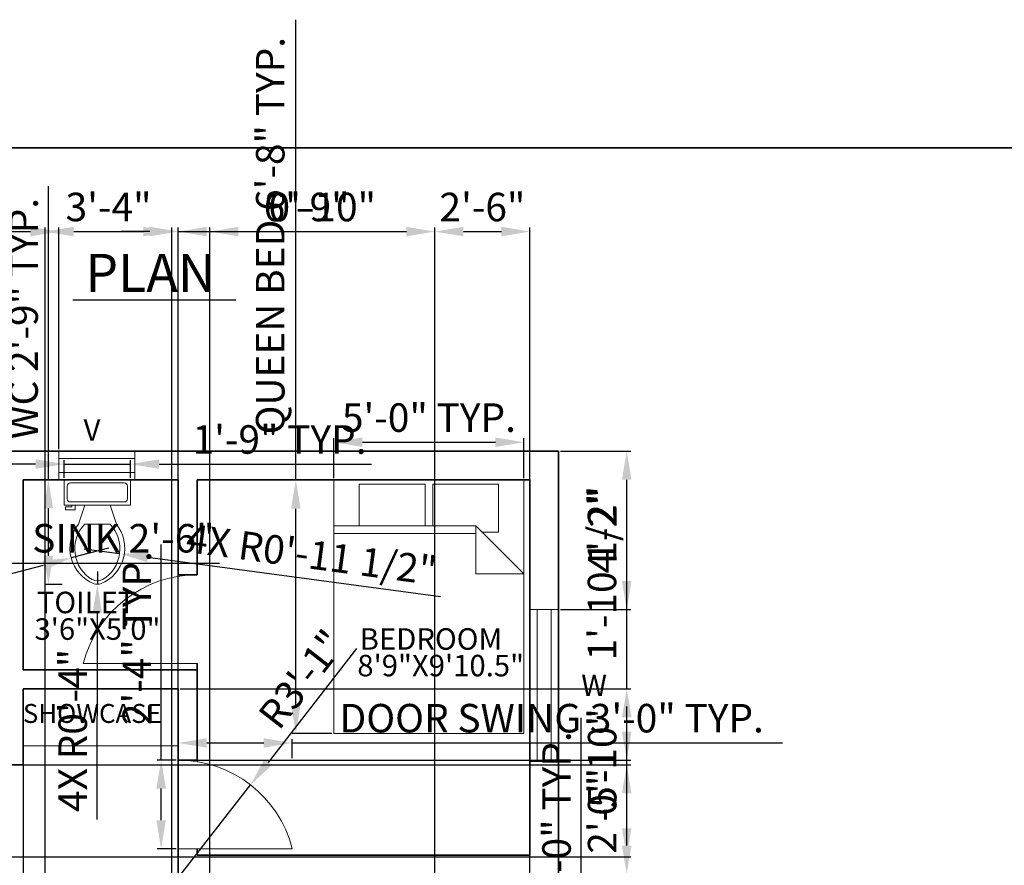
# Model space of a CAD drawing. Units: inches. Extents: x 1838 to 3181, y 1882 to 2430.
# Tile 3 of 4: x 2073 to 2384, y 2163 to 2430. Entities that reach past the tile are written whole.
import ezdxf

# ---------------------------------------------------------------- set-up
doc = ezdxf.new("R2010")
doc.units = ezdxf.units.IN
doc.linetypes.add('ACAD_ISO02W100', pattern=[15, 12, -3])
for name, color, linetype, lineweight in [('A-ANNO-TEXT', 7, 'Continuous', 18), ('A-ANNO-TITL', 6, 'Continuous', 25), ('A-ANNO-TTLB', 7, 'Continuous', 35), ('A-AREA-IDEN', 7, 'Continuous', 18), ('A-DOOR', 4, 'Continuous', 18), ('A-FLOR-CASE', 8, 'Continuous', 18), ('A-FLOR-FIXT', 9, 'Continuous', 18), ('A-FURN', 8, 'Continuous', 18), ('A-GLAZ', 11, 'Continuous', 18), ('A-WALL', 7, 'Continuous', 35), ('A-WALL-OVHD', 7, 'ACAD_ISO02W100', 18), ('S-ANNO-DIMS', 2, 'Continuous', 18)]:
    doc.layers.add(name, color=color, linetype=linetype, lineweight=lineweight)
doc.styles.get("Standard").update_dxf_attribs({"font": 'arial.ttf'})
doc.dimstyles.new('ISO-25', dxfattribs={"dimtxt": 9, "dimasz": 9, "dimexe": 1.25, "dimexo": 0.625, "dimgap": 2, "dimtad": 1, "dimdec": 1, "dimlunit": 4, "dimtxsty": 'Standard', "dimcen": 2.5, "dimadec": 0, "dimazin": 0, "dimtfac": 1, "dimtdec": 1, "dimtmove": 0, "dimatfit": 3, "dimfxl": 1, "dimarcsym": 0})

# ---------------------------------------------------------------- blocks, each defined once
blk = doc.blocks.new('Bed - Queen')
for p, q in [((0, -80.00003), (0, 0)), ((0, 0), (59.99999, 0)), ((59.99999, 0), (59.99999, -80.00003)), ((7.99999, -1.2), (28.79998, -1.2)), ((7.99999, -14.4), (7.99999, -1.2)), ((28.79998, -1.2), (28.79998, -14.4)), ((31.19999, -1.2), (51.99999, -1.2)), ((31.19999, -14.4), (31.19999, -1.2)), ((51.99999, -1.2), (51.99999, -16.4)), ((0, -14.4), (44.8, -14.4)), ((59.99999, -29.6), (44.8, -14.4)), ((44.8, -14.4), (44.8, -29.6)), ((44.8, -16.8), (0, -16.8)), ((51.99999, -16.4), (46.79936, -16.4)), ((44.8, -29.6), (59.99999, -29.6)), ((59.99999, -80.00003), (0, -80.00003))]:
    blk.add_line(p, q)
blk = doc.blocks.new('Toilet - top')
for p, q in [((9.5, -6), (9.5, -2)), ((-10, -8.5), (-8, -8.5)), ((-10, -9.5), (-10, -8.5)), ((-8, -8.5), (-8, -8)), ((-7, -8), (-7, -9.5)), ((-4, -8), (-6, -14)), ((4, -8), (6, -14)), ((-7, -9.5), (-10, -9.5)), ((4, -14), (-4, -14))]:
    blk.add_line(p, q)
blk.add_lwpolyline([(10.5, -8), (10.5, 0), (-10.5, 0), (-10.5, -8)], close=True)
for points in [[(-9.5, -2), (-9.5, -6)], [(8.5, -1), (-8.5, -1)], [(-8.5, -7), (8.5, -7)]]:
    blk.add_lwpolyline(points)
for centre, radius, start, end in [((-8.62, -1.88), 0.884, 81.8699, 188.1301), ((8.62, -1.88), 0.884, 351.8699, 98.1301), ((-8.62, -6.12), 0.884, 171.8699, 278.1301), ((8.62, -6.12), 0.884, 261.8699, 8.1301), ((3.52, -21.58), 12.17, 141.4691, 247.9714), ((4.2, -21.82), 11.33, 136.3677, 238.9468), ((-3.52, -21.58), 12.17, 292.0284, 38.5307), ((-4.2, -21.82), 11.33, 301.053, 43.6321), ((0, -27.88), 4, 245.7318, 294.2682), ((0, -29), 4, 254.8605, 285.1395)]:
    blk.add_arc(centre, radius, start, end)
blk = doc.blocks.new('WIN-48')
for p, q in [((0, 48), (9, 48)), ((2.25, 48), (2.25, 0)), ((6.75, 48), (6.75, 0)), ((0, 0), (9, 0))]:
    blk.add_line(p, q)
blk = doc.blocks.new('VENT-24')
for p, q in [((0, 24), (9, 24)), ((2.25, 24), (2.25, 0)), ((6.75, 24), (6.75, 0)), ((0, 0), (9, 0))]:
    blk.add_line(p, q)
blk = doc.blocks.new('DOOR-SWING-36')
blk.add_line((0, 0), (36, 0))
blk.add_arc((0, -9.14), 37.14, 14.25, 90)
blk = doc.blocks.new('*D23')
at = {"layer": 'Defpoints', "color": 0, "transparency": 16777216}
for p in [(2243.53, 2082.46), (2250.73, 2082.46), (2243.53, 2034.46)]:
    blk.add_point(p, dxfattribs=at)
at = {"layer": 'S-ANNO-DIMS', "color": 0, "lineweight": -2, "transparency": 16777216}
for p, q in [((2250.73, 2082.46), (2250.73, 2209.34)), ((2244.16, 2082.46), (2251.98, 2082.46)), ((2250.73, 2043.46), (2250.73, 2073.46)), ((2244.16, 2034.46), (2251.98, 2034.46))]:
    blk.add_line(p, q, dxfattribs=at)
at = {"layer": 'S-ANNO-DIMS', "color": 0, "transparency": 16777216}
for points in [[(2249.23, 2073.46), (2252.23, 2073.46), (2250.73, 2082.46)], [(2249.23, 2043.46), (2252.23, 2043.46), (2250.73, 2034.46)]]:
    blk.add_solid(points, dxfattribs=at)
at = {"layer": 'S-ANNO-DIMS', "color": 0, "transparency": 16777216, "insert": (2244.08, 2150.4), "char_height": 9, "attachment_point": 5, "rotation": 90}
blk.add_mtext('WINDOW 4\'-0" TYP.', dxfattribs=at)
blk = doc.blocks.new('*D27')
at = {"layer": 'Defpoints', "color": 0, "transparency": 16777216}
for p in [(2159.53, 2201.36), (2123.53, 2195.96), (2159.53, 2195.96)]:
    blk.add_point(p, dxfattribs=at)
at = {"layer": 'S-ANNO-DIMS', "color": 0, "lineweight": -2, "transparency": 16777216}
for p, q in [((2123.53, 2196.58), (2123.53, 2202.61)), ((2132.53, 2201.36), (2150.53, 2201.36)), ((2159.53, 2196.58), (2159.53, 2202.61)), ((2159.53, 2201.36), (2314.26, 2201.36))]:
    blk.add_line(p, q, dxfattribs=at)
at = {"layer": 'S-ANNO-DIMS', "color": 0, "transparency": 16777216}
for points in [[(2132.53, 2202.86), (2132.53, 2199.86), (2123.53, 2201.36)], [(2150.53, 2202.86), (2150.53, 2199.86), (2159.53, 2201.36)]]:
    blk.add_solid(points, dxfattribs=at)
at = {"layer": 'S-ANNO-DIMS', "color": 0, "transparency": 16777216, "insert": (2241.4, 2208.02), "char_height": 9, "attachment_point": 5}
blk.add_mtext('DOOR SWING 3\'-0" TYP.', dxfattribs=at)
blk = doc.blocks.new('*D28')
at = {"layer": 'Defpoints', "color": 0, "transparency": 16777216}
for p in [(2118.13, 2195.96), (2123.53, 2195.96), (2123.53, 2167.96)]:
    blk.add_point(p, dxfattribs=at)
at = {"layer": 'S-ANNO-DIMS', "color": 0, "lineweight": -2, "transparency": 16777216}
for p, q in [((2118.13, 2195.96), (2118.13, 2263.97)), ((2122.91, 2195.96), (2116.88, 2195.96)), ((2118.13, 2176.96), (2118.13, 2186.96)), ((2122.91, 2167.96), (2116.88, 2167.96))]:
    blk.add_line(p, q, dxfattribs=at)
at = {"layer": 'S-ANNO-DIMS', "color": 0, "transparency": 16777216}
for points in [[(2116.63, 2186.96), (2119.63, 2186.96), (2118.13, 2195.96)], [(2116.63, 2176.96), (2119.63, 2176.96), (2118.13, 2167.96)]]:
    blk.add_solid(points, dxfattribs=at)
at = {"layer": 'S-ANNO-DIMS', "color": 0, "transparency": 16777216, "insert": (2111.61, 2234.46), "char_height": 9, "attachment_point": 5, "rotation": 90}
blk.add_mtext('2\'-4" TYP.', dxfattribs=at)
blk = doc.blocks.new('*D29')
at = {"layer": 'Defpoints', "color": 0, "transparency": 16777216}
for p in [(2160.65, 2284.32), (2172.65, 2284.32), (2172.65, 2204.32)]:
    blk.add_point(p, dxfattribs=at)
at = {"layer": 'S-ANNO-DIMS', "color": 0, "lineweight": -2, "transparency": 16777216}
for p, q in [((2160.65, 2284.32), (2160.65, 2429.71)), ((2172.02, 2284.32), (2159.4, 2284.32)), ((2160.65, 2213.32), (2160.65, 2275.32)), ((2172.02, 2204.32), (2159.4, 2204.32))]:
    blk.add_line(p, q, dxfattribs=at)
at = {"layer": 'S-ANNO-DIMS', "color": 0, "transparency": 16777216}
for points in [[(2159.15, 2275.32), (2162.15, 2275.32), (2160.65, 2284.32)], [(2159.15, 2213.32), (2162.15, 2213.32), (2160.65, 2204.32)]]:
    blk.add_solid(points, dxfattribs=at)
at = {"layer": 'S-ANNO-DIMS', "color": 0, "transparency": 16777216, "insert": (2153.72, 2361.52), "char_height": 9, "attachment_point": 5, "rotation": 90}
blk.add_mtext('QUEEN BED 6\'-8" TYP.', dxfattribs=at)
blk = doc.blocks.new('*D30')
at = {"layer": 'Defpoints', "color": 0, "transparency": 16777216}
for p in [(2232.65, 2296.32), (2172.65, 2284.32), (2232.65, 2284.32)]:
    blk.add_point(p, dxfattribs=at)
at = {"layer": 'S-ANNO-DIMS', "color": 0, "lineweight": -2, "transparency": 16777216}
for p, q in [((2172.65, 2284.95), (2172.65, 2297.57)), ((2232.65, 2284.95), (2232.65, 2297.57)), ((2181.65, 2296.32), (2223.65, 2296.32))]:
    blk.add_line(p, q, dxfattribs=at)
at = {"layer": 'S-ANNO-DIMS', "color": 0, "transparency": 16777216}
for points in [[(2181.65, 2297.82), (2181.65, 2294.82), (2172.65, 2296.32)], [(2223.65, 2297.82), (2223.65, 2294.82), (2232.65, 2296.32)]]:
    blk.add_solid(points, dxfattribs=at)
at = {"layer": 'S-ANNO-DIMS', "color": 0, "transparency": 16777216, "insert": (2202.65, 2302.92), "char_height": 9, "attachment_point": 5}
blk.add_mtext('5\'-0" TYP.', dxfattribs=at)
blk = doc.blocks.new('*D31')
at = {"layer": 'Defpoints', "color": 0, "transparency": 16777216}
for p in [(2082.53, 2284.46), (2087.49, 2284.46), (2087.49, 2251.41)]:
    blk.add_point(p, dxfattribs=at)
at = {"layer": 'S-ANNO-DIMS', "color": 0, "lineweight": -2, "transparency": 16777216}
for p, q in [((2082.53, 2284.46), (2082.53, 2377.12)), ((2086.87, 2284.46), (2081.28, 2284.46)), ((2082.53, 2260.41), (2082.53, 2275.46)), ((2086.87, 2251.41), (2081.28, 2251.41))]:
    blk.add_line(p, q, dxfattribs=at)
at = {"layer": 'S-ANNO-DIMS', "color": 0, "transparency": 16777216}
for points in [[(2081.03, 2275.46), (2084.03, 2275.46), (2082.53, 2284.46)], [(2081.03, 2260.41), (2084.03, 2260.41), (2082.53, 2251.41)]]:
    blk.add_solid(points, dxfattribs=at)
at = {"layer": 'S-ANNO-DIMS', "color": 0, "transparency": 16777216, "insert": (2075.88, 2335.29), "char_height": 9, "attachment_point": 5, "rotation": 90}
blk.add_mtext('WC 2\'-9" TYP.', dxfattribs=at)
blk = doc.blocks.new('*D32')
at = {"layer": 'Defpoints', "color": 0, "transparency": 16777216}
for p in [(2108.49, 2289.41), (2087.49, 2284.46), (2108.49, 2284.46)]:
    blk.add_point(p, dxfattribs=at)
at = {"layer": 'S-ANNO-DIMS', "color": 0, "lineweight": -2, "transparency": 16777216}
for p, q in [((2087.49, 2285.08), (2087.49, 2290.66)), ((2108.49, 2285.08), (2108.49, 2290.66)), ((2078.49, 2289.41), (2069.49, 2289.41)), ((2087.49, 2289.41), (2108.49, 2289.41)), ((2117.49, 2289.41), (2184.5, 2289.41))]:
    blk.add_line(p, q, dxfattribs=at)
at = {"layer": 'S-ANNO-DIMS', "color": 0, "transparency": 16777216}
for points in [[(2078.49, 2290.91), (2078.49, 2287.91), (2087.49, 2289.41)], [(2117.49, 2290.91), (2117.49, 2287.91), (2108.49, 2289.41)]]:
    blk.add_solid(points, dxfattribs=at)
at = {"layer": 'S-ANNO-DIMS', "color": 0, "transparency": 16777216, "insert": (2155.5, 2296.01), "char_height": 9, "attachment_point": 5}
blk.add_mtext('1\'-9" TYP.', dxfattribs=at)
blk = doc.blocks.new('*D37')
at = {"layer": 'Defpoints', "color": 0, "transparency": 16777216}
for p in [(2036.86, 2262.67), (2066.86, 2262.67), (2066.86, 2258.17)]:
    blk.add_point(p, dxfattribs=at)
at = {"layer": 'S-ANNO-DIMS', "color": 0, "lineweight": -2, "transparency": 16777216}
for p, q in [((2036.86, 2262.04), (2036.86, 2256.92)), ((2066.86, 2262.04), (2066.86, 2256.92)), ((2045.86, 2258.17), (2057.86, 2258.17)), ((2066.86, 2258.17), (2136.58, 2258.17))]:
    blk.add_line(p, q, dxfattribs=at)
at = {"layer": 'S-ANNO-DIMS', "color": 0, "transparency": 16777216}
for points in [[(2045.86, 2259.67), (2045.86, 2256.67), (2036.86, 2258.17)], [(2057.86, 2259.67), (2057.86, 2256.67), (2066.86, 2258.17)]]:
    blk.add_solid(points, dxfattribs=at)
at = {"layer": 'S-ANNO-DIMS', "color": 0, "transparency": 16777216, "insert": (2106.22, 2264.82), "char_height": 9, "attachment_point": 5}
blk.add_mtext('SINK 2\'-6"', dxfattribs=at)
blk = doc.blocks.new('*D42')
at = {"layer": 'Defpoints', "color": 0, "transparency": 16777216}
for p in [(2002.53, 2194.46), (2265.08, 2194.46), (2002.53, 2165.46)]:
    blk.add_point(p, dxfattribs=at)
at = {"layer": 'S-ANNO-DIMS', "color": 0, "lineweight": -2, "transparency": 16777216}
for p, q in [((2003.16, 2194.46), (2266.33, 2194.46)), ((2265.08, 2174.46), (2265.08, 2185.46)), ((2003.16, 2165.46), (2266.33, 2165.46))]:
    blk.add_line(p, q, dxfattribs=at)
at = {"layer": 'S-ANNO-DIMS', "color": 0, "transparency": 16777216}
for points in [[(2263.58, 2185.46), (2266.58, 2185.46), (2265.08, 2194.46)], [(2263.58, 2174.46), (2266.58, 2174.46), (2265.08, 2165.46)]]:
    blk.add_solid(points, dxfattribs=at)
at = {"layer": 'S-ANNO-DIMS', "color": 0, "transparency": 16777216, "insert": (2258.49, 2179.96), "char_height": 9, "attachment_point": 5, "rotation": 90}
blk.add_mtext('2\'-5"', dxfattribs=at)
blk = doc.blocks.new('*D46')
at = {"layer": 'Defpoints', "color": 0, "transparency": 16777216}
for p in [(2234.53, 2159.96), (2265.08, 2159.96), (2234.53, 2149.73)]:
    blk.add_point(p, dxfattribs=at)
at = {"layer": 'S-ANNO-DIMS', "color": 0, "lineweight": -2, "transparency": 16777216}
for p, q in [((2265.08, 2168.96), (2265.08, 2212.87)), ((2235.16, 2159.96), (2266.33, 2159.96)), ((2265.08, 2149.73), (2265.08, 2159.96)), ((2235.16, 2149.73), (2266.33, 2149.73)), ((2265.08, 2140.73), (2265.08, 2131.73))]:
    blk.add_line(p, q, dxfattribs=at)
at = {"layer": 'S-ANNO-DIMS', "color": 0, "transparency": 16777216}
for points in [[(2263.58, 2168.96), (2266.58, 2168.96), (2265.08, 2159.96)], [(2263.58, 2140.73), (2266.58, 2140.73), (2265.08, 2149.73)]]:
    blk.add_solid(points, dxfattribs=at)
at = {"layer": 'S-ANNO-DIMS', "color": 0, "transparency": 16777216, "insert": (2258.49, 2195.41), "char_height": 9, "attachment_point": 5, "rotation": 90}
blk.add_mtext('0\'-10"', dxfattribs=at)
blk = doc.blocks.new('*D47')
at = {"layer": 'Defpoints', "color": 0, "transparency": 16777216}
for p in [(2243.53, 2293.46), (2265.08, 2293.46), (2243.53, 2243.46)]:
    blk.add_point(p, dxfattribs=at)
at = {"layer": 'S-ANNO-DIMS', "color": 0, "lineweight": -2, "transparency": 16777216}
for p, q in [((2244.16, 2293.46), (2266.33, 2293.46)), ((2265.08, 2252.46), (2265.08, 2284.46)), ((2244.16, 2243.46), (2266.33, 2243.46))]:
    blk.add_line(p, q, dxfattribs=at)
at = {"layer": 'S-ANNO-DIMS', "color": 0, "transparency": 16777216}
for points in [[(2263.58, 2284.46), (2266.58, 2284.46), (2265.08, 2293.46)], [(2263.58, 2252.46), (2266.58, 2252.46), (2265.08, 2243.46)]]:
    blk.add_solid(points, dxfattribs=at)
at = {"layer": 'S-ANNO-DIMS', "color": 0, "transparency": 16777216, "insert": (2258.57, 2268.46), "char_height": 9, "attachment_point": 5, "rotation": 90}
blk.add_mtext('4\'-2"', dxfattribs=at)
blk = doc.blocks.new('*D48')
at = {"layer": 'Defpoints', "color": 0, "transparency": 16777216}
for p in [(2085.84, 2362.82), (1993.53, 2293.46), (2085.84, 2293.46)]:
    blk.add_point(p, dxfattribs=at)
at = {"layer": 'S-ANNO-DIMS', "color": 0, "lineweight": -2, "transparency": 16777216}
for p, q in [((1993.53, 2294.08), (1993.53, 2364.07)), ((2002.53, 2362.82), (2076.84, 2362.82)), ((2085.84, 2294.08), (2085.84, 2364.07))]:
    blk.add_line(p, q, dxfattribs=at)
at = {"layer": 'S-ANNO-DIMS', "color": 0, "transparency": 16777216}
for points in [[(2002.53, 2364.32), (2002.53, 2361.32), (1993.53, 2362.82)], [(2076.84, 2364.32), (2076.84, 2361.32), (2085.84, 2362.82)]]:
    blk.add_solid(points, dxfattribs=at)
at = {"layer": 'S-ANNO-DIMS', "color": 0, "transparency": 16777216, "insert": (2039.69, 2369.47), "char_height": 9, "attachment_point": 5}
blk.add_mtext('7\'-8 1/2"', dxfattribs=at)
blk = doc.blocks.new('*D49')
at = {"layer": 'Defpoints', "color": 0, "transparency": 16777216}
for p in [(2133.53, 2362.82), (2123.53, 1939.46), (2133.53, 1939.46)]:
    blk.add_point(p, dxfattribs=at)
at = {"layer": 'S-ANNO-DIMS', "color": 0, "lineweight": -2, "transparency": 16777216}
for p, q in [((2114.53, 2362.82), (2105.53, 2362.82)), ((2123.53, 1940.08), (2123.53, 2364.07)), ((2123.53, 2362.82), (2133.53, 2362.82)), ((2133.53, 1940.08), (2133.53, 2364.07)), ((2142.53, 2362.82), (2186.45, 2362.82))]:
    blk.add_line(p, q, dxfattribs=at)
at = {"layer": 'S-ANNO-DIMS', "color": 0, "transparency": 16777216}
for points in [[(2114.53, 2364.32), (2114.53, 2361.32), (2123.53, 2362.82)], [(2142.53, 2364.32), (2142.53, 2361.32), (2133.53, 2362.82)]]:
    blk.add_solid(points, dxfattribs=at)
at = {"layer": 'S-ANNO-DIMS', "color": 0, "transparency": 16777216, "insert": (2168.99, 2369.41), "char_height": 9, "attachment_point": 5}
blk.add_mtext('0\'-10"', dxfattribs=at)
blk = doc.blocks.new('*D50')
at = {"layer": 'Defpoints', "color": 0, "transparency": 16777216}
for p in [(2204.53, 2362.82), (2123.53, 1999.46), (2204.53, 1999.46)]:
    blk.add_point(p, dxfattribs=at)
at = {"layer": 'S-ANNO-DIMS', "color": 0, "lineweight": -2, "transparency": 16777216}
for p, q in [((2123.53, 2000.08), (2123.53, 2364.07)), ((2132.53, 2362.82), (2195.53, 2362.82)), ((2204.53, 2000.08), (2204.53, 2364.07))]:
    blk.add_line(p, q, dxfattribs=at)
at = {"layer": 'S-ANNO-DIMS', "color": 0, "transparency": 16777216}
for points in [[(2132.53, 2364.32), (2132.53, 2361.32), (2123.53, 2362.82)], [(2195.53, 2364.32), (2195.53, 2361.32), (2204.53, 2362.82)]]:
    blk.add_solid(points, dxfattribs=at)
at = {"layer": 'S-ANNO-DIMS', "color": 0, "transparency": 16777216, "insert": (2164.03, 2369.41), "char_height": 9, "attachment_point": 5}
blk.add_mtext('6\'-9"', dxfattribs=at)
blk = doc.blocks.new('*D51')
at = {"layer": 'Defpoints', "color": 0, "transparency": 16777216}
for p in [(2234.53, 2362.82), (2204.53, 1999.46), (2234.53, 1999.46)]:
    blk.add_point(p, dxfattribs=at)
at = {"layer": 'S-ANNO-DIMS', "color": 0, "lineweight": -2, "transparency": 16777216}
for p, q in [((2204.53, 2000.08), (2204.53, 2364.07)), ((2213.53, 2362.82), (2225.53, 2362.82)), ((2234.53, 2000.08), (2234.53, 2364.07))]:
    blk.add_line(p, q, dxfattribs=at)
at = {"layer": 'S-ANNO-DIMS', "color": 0, "transparency": 16777216}
for points in [[(2213.53, 2364.32), (2213.53, 2361.32), (2204.53, 2362.82)], [(2225.53, 2364.32), (2225.53, 2361.32), (2234.53, 2362.82)]]:
    blk.add_solid(points, dxfattribs=at)
at = {"layer": 'S-ANNO-DIMS', "color": 0, "transparency": 16777216, "insert": (2219.53, 2369.41), "char_height": 9, "attachment_point": 5}
blk.add_mtext('2\'-6"', dxfattribs=at)
blk = doc.blocks.new('*D53')
at = {"layer": 'Defpoints', "color": 0, "transparency": 16777216}
for p in [(2121.53, 2362.82), (2081.53, 1999.46), (2121.53, 1999.46)]:
    blk.add_point(p, dxfattribs=at)
at = {"layer": 'S-ANNO-DIMS', "color": 0, "lineweight": -2, "transparency": 16777216}
for p, q in [((2081.53, 2000.08), (2081.53, 2364.07)), ((2090.53, 2362.82), (2112.53, 2362.82)), ((2121.53, 2000.08), (2121.53, 2364.07))]:
    blk.add_line(p, q, dxfattribs=at)
at = {"layer": 'S-ANNO-DIMS', "color": 0, "transparency": 16777216}
for points in [[(2090.53, 2364.32), (2090.53, 2361.32), (2081.53, 2362.82)], [(2112.53, 2364.32), (2112.53, 2361.32), (2121.53, 2362.82)]]:
    blk.add_solid(points, dxfattribs=at)
at = {"layer": 'S-ANNO-DIMS', "color": 0, "transparency": 16777216, "insert": (2101.53, 2369.42), "char_height": 9, "attachment_point": 5}
blk.add_mtext('3\'-4"', dxfattribs=at)
blk = doc.blocks.new('*D55')
at = {"layer": 'Defpoints', "color": 0, "transparency": 16777216}
for p in [(2068.53, 2194.46), (2074.53, 2194.46), (2074.53, 1908.91)]:
    blk.add_point(p, dxfattribs=at)
at = {"layer": 'S-ANNO-DIMS', "color": 0, "lineweight": -2, "transparency": 16777216}
for p, q in [((2068.53, 2193.83), (2068.53, 1907.66)), ((2074.53, 2193.83), (2074.53, 1907.66)), ((2059.53, 1908.91), (2050.53, 1908.91)), ((2068.53, 1908.91), (2074.53, 1908.91)), ((2083.53, 1908.91), (2120.46, 1908.91))]:
    blk.add_line(p, q, dxfattribs=at)
at = {"layer": 'S-ANNO-DIMS', "color": 0, "transparency": 16777216}
for points in [[(2059.53, 1910.41), (2059.53, 1907.41), (2068.53, 1908.91)], [(2083.53, 1910.41), (2083.53, 1907.41), (2074.53, 1908.91)]]:
    blk.add_solid(points, dxfattribs=at)
at = {"layer": 'S-ANNO-DIMS', "color": 0, "transparency": 16777216, "insert": (2106.5, 1915.5), "char_height": 9, "attachment_point": 5}
blk.add_mtext('0\'-6"', dxfattribs=at)
blk = doc.blocks.new('*D56')
at = {"layer": 'Defpoints', "color": 0, "transparency": 16777216}
for p in [(2074.53, 2218.46), (2123.53, 2218.46), (2123.53, 1908.91)]:
    blk.add_point(p, dxfattribs=at)
at = {"layer": 'S-ANNO-DIMS', "color": 0, "lineweight": -2, "transparency": 16777216}
for p, q in [((2074.53, 2217.83), (2074.53, 1907.66)), ((2123.53, 2217.83), (2123.53, 1907.66)), ((2083.53, 1908.91), (2114.53, 1908.91))]:
    blk.add_line(p, q, dxfattribs=at)
at = {"layer": 'S-ANNO-DIMS', "color": 0, "transparency": 16777216}
for points in [[(2083.53, 1910.41), (2083.53, 1907.41), (2074.53, 1908.91)], [(2114.53, 1910.41), (2114.53, 1907.41), (2123.53, 1908.91)]]:
    blk.add_solid(points, dxfattribs=at)
at = {"layer": 'S-ANNO-DIMS', "color": 0, "transparency": 16777216, "insert": (2099.03, 1915.42), "char_height": 9, "attachment_point": 5}
blk.add_mtext('4\'-1"', dxfattribs=at)
blk = doc.blocks.new('*D57')
at = {"layer": 'Defpoints', "color": 0, "transparency": 16777216}
for p in [(2123.53, 2218.46), (2265.08, 2218.46), (2123.53, 2195.96)]:
    blk.add_point(p, dxfattribs=at)
at = {"layer": 'S-ANNO-DIMS', "color": 0, "lineweight": -2, "transparency": 16777216}
for p, q in [((2265.08, 2218.46), (2265.08, 2282.5)), ((2124.16, 2218.46), (2266.33, 2218.46)), ((2265.08, 2204.96), (2265.08, 2209.46)), ((2124.16, 2195.96), (2266.33, 2195.96))]:
    blk.add_line(p, q, dxfattribs=at)
at = {"layer": 'S-ANNO-DIMS', "color": 0, "transparency": 16777216}
for points in [[(2263.58, 2209.46), (2266.58, 2209.46), (2265.08, 2218.46)], [(2263.58, 2204.96), (2266.58, 2204.96), (2265.08, 2195.96)]]:
    blk.add_solid(points, dxfattribs=at)
at = {"layer": 'S-ANNO-DIMS', "color": 0, "transparency": 16777216, "insert": (2258.43, 2254.98), "char_height": 9, "attachment_point": 5, "rotation": 90}
blk.add_mtext('1\'-10 1/2"', dxfattribs=at)
blk = doc.blocks.new('*D72')
at = {"layer": 'Defpoints', "color": 0, "transparency": 16777216}
for p in [(2146.34, 2188.13), (2123.53, 2158.81)]:
    blk.add_point(p, dxfattribs=at)
at = {"layer": 'S-ANNO-DIMS', "color": 0, "lineweight": -2, "transparency": 16777216}
for p, q in [((2179.82, 2231.18), (2151.86, 2195.24)), ((2123.53, 2158.81), (2146.34, 2188.13))]:
    blk.add_line(p, q, dxfattribs=at)
at = {"layer": 'S-ANNO-DIMS', "color": 0, "transparency": 16777216}
blk.add_solid([(2150.68, 2196.16), (2153.05, 2194.32), (2146.34, 2188.13)], dxfattribs=at)
at = {"layer": 'S-ANNO-DIMS', "color": 0, "transparency": 16777216, "insert": (2163.4, 2220.81), "char_height": 9, "attachment_point": 5, "rotation": 52.1256}
blk.add_mtext('R3\'-1"', dxfattribs=at)
blk = doc.blocks.new('*D74')
at = {"layer": 'Defpoints', "color": 0, "transparency": 16777216}
for p in [(2101.51, 2262.88), (2089.74, 2259.78)]:
    blk.add_point(p, dxfattribs=at)
at = {"layer": 'S-ANNO-DIMS', "color": 0, "lineweight": -2, "transparency": 16777216}
for p, q in [((2101.51, 2262.88), (2089.74, 2259.78)), ((2017.94, 2240.92), (2081.04, 2257.5))]:
    blk.add_line(p, q, dxfattribs=at)
at = {"layer": 'S-ANNO-DIMS', "color": 0, "transparency": 16777216}
blk.add_solid([(2080.65, 2258.95), (2081.42, 2256.05), (2089.74, 2259.78)], dxfattribs=at)
at = {"layer": 'S-ANNO-DIMS', "color": 0, "transparency": 16777216, "insert": (2043.46, 2254.44), "char_height": 9, "attachment_point": 5, "rotation": 14.7211}
blk.add_mtext('4X R1\'-0"', dxfattribs=at)
blk = doc.blocks.new('*D75')
at = {"layer": 'Defpoints', "color": 0, "transparency": 16777216}
for p in [(2093.79, 2262.64), (2105.02, 2261.13)]:
    blk.add_point(p, dxfattribs=at)
at = {"layer": 'S-ANNO-DIMS', "color": 0, "lineweight": -2, "transparency": 16777216}
for p, q in [((2093.79, 2262.64), (2105.02, 2261.13)), ((2206.31, 2247.51), (2113.94, 2259.93))]:
    blk.add_line(p, q, dxfattribs=at)
at = {"layer": 'S-ANNO-DIMS', "color": 0, "transparency": 16777216}
blk.add_solid([(2114.14, 2261.42), (2113.74, 2258.44), (2105.02, 2261.13)], dxfattribs=at)
at = {"layer": 'S-ANNO-DIMS', "color": 0, "transparency": 16777216, "insert": (2165.47, 2259.72), "char_height": 9, "attachment_point": 5, "rotation": 352.3432}
blk.add_mtext('4X R0\'-11 1/2"', dxfattribs=at)
blk = doc.blocks.new('*D76')
at = {"layer": 'Defpoints', "color": 0, "transparency": 16777216}
for p in [(2097.99, 2255.46), (2097.99, 2251.46)]:
    blk.add_point(p, dxfattribs=at)
at = {"layer": 'S-ANNO-DIMS', "color": 0, "lineweight": -2, "transparency": 16777216}
for p, q in [((2097.99, 2255.46), (2097.99, 2251.46)), ((2097.98, 2177.22), (2097.99, 2242.46))]:
    blk.add_line(p, q, dxfattribs=at)
at = {"layer": 'S-ANNO-DIMS', "color": 0, "transparency": 16777216}
blk.add_solid([(2096.49, 2242.46), (2099.49, 2242.46), (2097.99, 2251.46)], dxfattribs=at)
at = {"layer": 'S-ANNO-DIMS', "color": 0, "transparency": 16777216, "insert": (2091.39, 2205.34), "char_height": 9, "attachment_point": 5, "rotation": 89.9946}
blk.add_mtext('4X R0\'-4"', dxfattribs=at)

msp = doc.modelspace()

# ---------------------------------------------------------------- linework, layer by layer
at = {"layer": 'A-ANNO-TITL'}
msp.add_line((2090.21, 2341.27), (2141.65, 2341.27), dxfattribs=at)
at = {"layer": 'A-ANNO-TTLB'}
msp.add_lwpolyline([(1905.37, 2389.23), (3180.85, 2389.23), (3180.85, 1893.51), (1905.37, 1893.51)], close=True, dxfattribs=at)
at = {"layer": 'A-FLOR-CASE'}
msp.add_line((2074.53, 2200.46), (2123.53, 2200.46), dxfattribs=at)
at = {"layer": 'A-WALL'}
for p, q in [((1993.53, 2293.46), (2243.53, 2293.46)), ((2243.53, 2293.46), (2243.53, 1930.46)), ((2074.53, 2284.46), (2074.53, 2224.46)), ((2074.53, 2284.46), (2123.53, 2284.46)), ((2123.53, 2284.46), (2123.53, 2254.46)), ((2129.53, 2284.46), (2129.53, 2254.46)), ((2129.53, 2284.46), (2234.53, 2284.46)), ((2234.53, 2284.46), (2234.53, 2165.96)), ((2123.53, 2254.46), (2129.53, 2254.46)), ((2129.53, 2226.46), (2129.53, 2195.96)), ((2074.53, 2224.46), (2129.53, 2224.46)), ((2074.53, 2218.46), (2123.53, 2218.46)), ((2074.53, 2218.46), (2074.53, 2194.46)), ((2123.53, 2218.46), (2123.53, 2195.96)), ((2068.53, 2194.46), (2074.53, 2194.46)), ((2123.53, 2195.96), (2129.53, 2195.96)), ((2129.53, 2195.46), (2129.61, 2195.46)), ((2123.53, 2167.96), (2123.53, 2157.96)), ((2129.53, 2167.96), (2129.53, 2165.96)), ((2129.53, 2165.96), (2234.53, 2165.96))]:
    msp.add_line(p, q, dxfattribs=at)
at = {"layer": 'A-WALL-OVHD'}
msp.add_line((2030.53, 2194.46), (2074.53, 2194.46), dxfattribs=at)

# ---------------------------------------------------------------- block references
at = {"layer": 'A-DOOR', "extrusion": (0, 0, -1), "zscale": -1}
msp.add_blockref('DOOR-SWING-36', (-2129.53, 2226.46), dxfattribs=at)
at = {"layer": 'A-DOOR'}
msp.add_blockref('DOOR-SWING-36', (2123.53, 2167.96), dxfattribs=at)
at = {"layer": 'A-FLOR-FIXT'}
msp.add_blockref('Toilet - top', (2097.99, 2284.46), dxfattribs=at)
at = {"layer": 'A-FURN'}
msp.add_blockref('Bed - Queen', (2172.65, 2284.32), dxfattribs=at)
at = {"layer": 'A-GLAZ'}
for name, p, rotation in [('VENT-24', (2109.84, 2284.46), 90.00000000000641), ('WIN-48', (2243.53, 2243.46), 180)]:
    msp.add_blockref(name, p, dxfattribs=dict(at, rotation=rotation))

# ---------------------------------------------------------------- texts
at = {"layer": 'A-ANNO-TEXT'}
for s, height, p in [('V', 6.78, (2093.64, 2296.78)), ('W', 6.78, (2250.72, 2216.17)), ('SHOWCASE', 5.979, (2074.5, 2207.69))]:
    msp.add_text(s, height=height, dxfattribs=at).set_placement(p)
at = {"layer": 'A-ANNO-TITL'}
msp.add_text('PLAN', height=12, dxfattribs=at).set_placement((2094.19, 2343.79))
at = {"layer": 'A-AREA-IDEN'}
for s, height, p in [('TOILET', 6.784, (2078.88, 2242.33)), (' 3\'6"X5\'0"', 6.784, (2076.07, 2233.93)), ('BEDROOM', 6.784, (2180.78, 2230.8)), (' 8\'9"X9\'10.5"', 6.7841, (2177.97, 2222.4))]:
    msp.add_text(s, height=height, dxfattribs=at).set_placement(p)

# ---------------------------------------------------------------- dimensions: what is measured, and where the dimension line sits
at = {"layer": 'S-ANNO-DIMS'}
for base, p1, p2, text, picture, middle in [((2160.65, 2284.32), (2172.65, 2204.32), (2172.65, 2284.32), 'QUEEN BED <> TYP.', '*D29', (2153.72, 2361.52)), ((2082.5334, 2284.4559), (2087.4904, 2251.4097), (2087.4904, 2284.4559), 'WC <> TYP.', '*D31', (2075.8799, 2335.2898)), ((2118.13, 2195.96), (2123.53, 2167.96), (2123.53, 2195.96), '<> TYP.', '*D28', (2111.61, 2234.46)), ((2250.73, 2082.46), (2243.53, 2034.46), (2243.53, 2082.46), 'WINDOW <> TYP.', '*D23', (2244.08, 2150.4))]:
    dim = msp.add_linear_dim(base=base, p1=p1, p2=p2, angle=90, text=text, dimstyle='ISO-25', override={"dimdec": 1, "dimlfac": 1, "dimrnd": 0, "dimzin": 1, "dimdsep": 46, "dimlunit": 4, "dimfrac": 2}, dxfattribs=at)
    dim.commit()
    dim.dimension.update_dxf_attribs({"geometry": picture, "text_midpoint": middle})
for base, p1, p2, picture, middle in [((2085.84, 2362.82), (1993.53, 2293.46), (2085.84, 2293.46), '*D48', (2039.69, 2369.47)), ((2121.53, 2362.82), (2081.53, 1999.46), (2121.53, 1999.46), '*D53', (2101.53, 2369.42)), ((2133.53, 2362.82), (2123.53, 1939.46), (2133.53, 1939.46), '*D49', (2168.99, 2369.41)), ((2204.53, 2362.82), (2123.53, 1999.46), (2204.53, 1999.46), '*D50', (2164.03, 2369.41)), ((2234.53, 2362.82), (2204.53, 1999.46), (2234.53, 1999.46), '*D51', (2219.53, 2369.41)), ((2123.53, 1908.91), (2074.53, 2218.46), (2123.53, 2218.46), '*D56', (2099.03, 1915.42)), ((2074.53, 1908.91), (2068.53, 2194.46), (2074.53, 2194.46), '*D55', (2106.5, 1915.5))]:
    dim = msp.add_linear_dim(base=base, p1=p1, p2=p2, dimstyle='ISO-25', override={"dimdec": 1, "dimlfac": 1, "dimrnd": 0, "dimzin": 1, "dimdsep": 46, "dimlunit": 4, "dimfrac": 2}, dxfattribs=at)
    dim.commit()
    dim.dimension.update_dxf_attribs({"geometry": picture, "text_midpoint": middle})
for base, p1, p2, text, picture, middle in [((2232.65, 2296.32), (2172.65, 2284.32), (2232.65, 2284.32), '<> TYP.', '*D30', (2202.65, 2302.92)), ((2108.49, 2289.41), (2087.49, 2284.46), (2108.49, 2284.46), '<> TYP.', '*D32', (2155.5, 2296.01)), ((2066.86, 2258.17), (2036.86, 2262.67), (2066.86, 2262.67), 'SINK <>', '*D37', (2106.22, 2264.82)), ((2159.53, 2201.36), (2123.53, 2195.96), (2159.53, 2195.96), 'DOOR SWING <> TYP.', '*D27', (2241.4, 2208.02))]:
    dim = msp.add_linear_dim(base=base, p1=p1, p2=p2, text=text, dimstyle='ISO-25', override={"dimdec": 1, "dimlfac": 1, "dimrnd": 0, "dimzin": 1, "dimdsep": 46, "dimlunit": 4, "dimfrac": 2}, dxfattribs=at)
    dim.commit()
    dim.dimension.update_dxf_attribs({"geometry": picture, "text_midpoint": middle})
for base, p1, p2, picture, middle in [((2265.08, 2293.46), (2243.53, 2243.46), (2243.53, 2293.46), '*D47', (2258.57, 2268.46)), ((2265.08, 2218.46), (2123.53, 2195.96), (2123.53, 2218.46), '*D57', (2258.43, 2254.98)), ((2265.08, 2159.96), (2234.53, 2149.73), (2234.53, 2159.96), '*D46', (2258.49, 2195.41)), ((2265.08, 2194.46), (2002.53, 2165.46), (2002.53, 2194.46), '*D42', (2258.49, 2179.96))]:
    dim = msp.add_linear_dim(base=base, p1=p1, p2=p2, angle=90, dimstyle='ISO-25', override={"dimdec": 1, "dimlfac": 1, "dimrnd": 0, "dimzin": 1, "dimdsep": 46, "dimlunit": 4, "dimfrac": 2}, dxfattribs=at)
    dim.commit()
    dim.dimension.update_dxf_attribs({"geometry": picture, "text_midpoint": middle})
for center, mpoint, picture, middle in [((2093.79, 2262.64), (2105.02, 2261.13), '*D75', (2165.47, 2259.72)), ((2101.51, 2262.88), (2089.74, 2259.78), '*D74', (2043.46, 2254.44)), ((2097.99, 2255.46), (2097.99, 2251.46), '*D76', (2091.39, 2205.34))]:
    dim = msp.add_radius_dim(center=center, mpoint=mpoint, text='4X <>', dimstyle='ISO-25', override={"dimdec": 1, "dimlfac": 1, "dimrnd": 0, "dimzin": 1, "dimdsep": 46, "dimlunit": 4, "dimfrac": 2}, dxfattribs=at)
    dim.commit()
    dim.dimension.update_dxf_attribs({"geometry": picture, "text_midpoint": middle})
dim = msp.add_radius_dim(center=(2123.53, 2158.81), mpoint=(2146.34, 2188.13), dimstyle='ISO-25', override={"dimdec": 1, "dimlfac": 1, "dimrnd": 0, "dimzin": 1, "dimdsep": 46, "dimlunit": 4, "dimfrac": 2}, dxfattribs=at)
dim.commit()
dim.dimension.update_dxf_attribs({"geometry": '*D72', "text_midpoint": (2163.4, 2220.81)})

doc.saveas('drawing.dxf')
